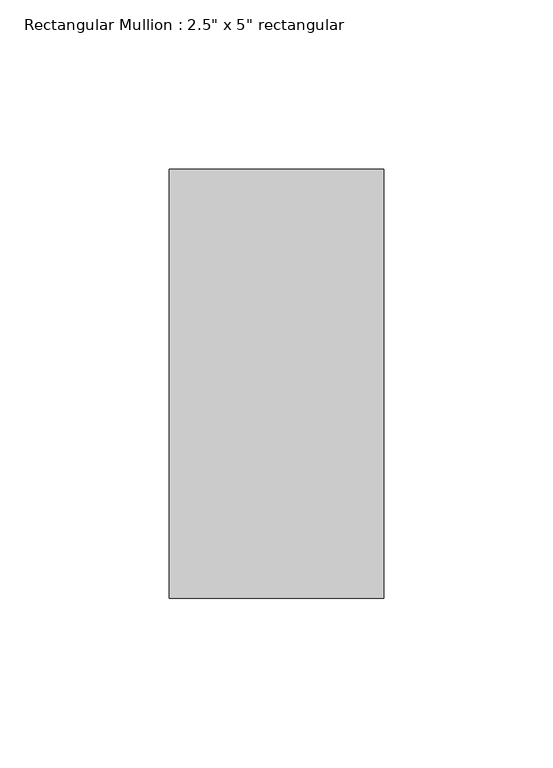
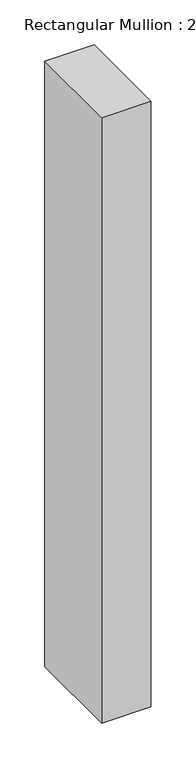
"""IFC4 building model written with IfcOpenShell, lengths in millimetres: member geometry."""

from ifc_helpers import new_model, si_unit, frame, origin, place, context, project, spatial, polyline, outline, extrude, source, transform, mapped, element, save


def member_e9605c56(model_context):
    return source(origin(), model_context, "Body", "SweptSolid", [
        extrude(outline(polyline([(0.0, 63.5), (0.0, -63.5), (-63.5, -63.5), (-63.5, 63.5), (0.0, 63.5)])), frame((0.0, 0.0, -825.5), z_axis=(0.0, 0.0, 1.0), x_axis=(1.0, 0.0, 0.0)), (0.0, 0.0, 1.0), 825.5),
    ])


if __name__ == "__main__":
    model = new_model("IFC4")
    model_context = context("Model", 3, world=origin())
    ifc_project = project(units=[si_unit("LENGTHUNIT", "METRE", prefix="MILLI")], contexts=[model_context])
    site = spatial("IfcSite", under=ifc_project)
    building = spatial("IfcBuilding", under=site)
    placement = place(None, origin())
    member_shape = member_e9605c56(model_context)
    element("IfcMember", 1, ObjectType="Rectangular Mullion : 2.5\" x 5\" rectangular", at=placement, inside=building, context=model_context, shape_type="MappedRepresentation", body=[
        mapped(member_shape, transform((0.0, 0.0, 0.0), x_axis=(1.0, 0.0, 0.0), y_axis=(0.0, 1.0, 0.0), z_axis=(0.0, 0.0, 1.0))),
    ])
    save(model, "model.ifc")

# Revit data of these elements
# Type "Rectangular Mullion : 2.5\" x 5\" rectangular"
#   built-in parameter 1007304 = 0.416667 (stored number, unit not read)
#   built-in parameter 1007301 = 0.104167 (stored number, unit not read)
#   built-in parameter 1007300 = 0.104167 (stored number, unit not read)
# Element 1 (IfcMember, "Rectangular Mullion : 2.5\" x 5\" rectangular")
#   Materials on its faces: "Aluminum"
# Materials
#   "Aluminum": class "Metal", colour RGB 247 247 247, transparency 0, Description = "Aluminum 6061", Cost = 0
